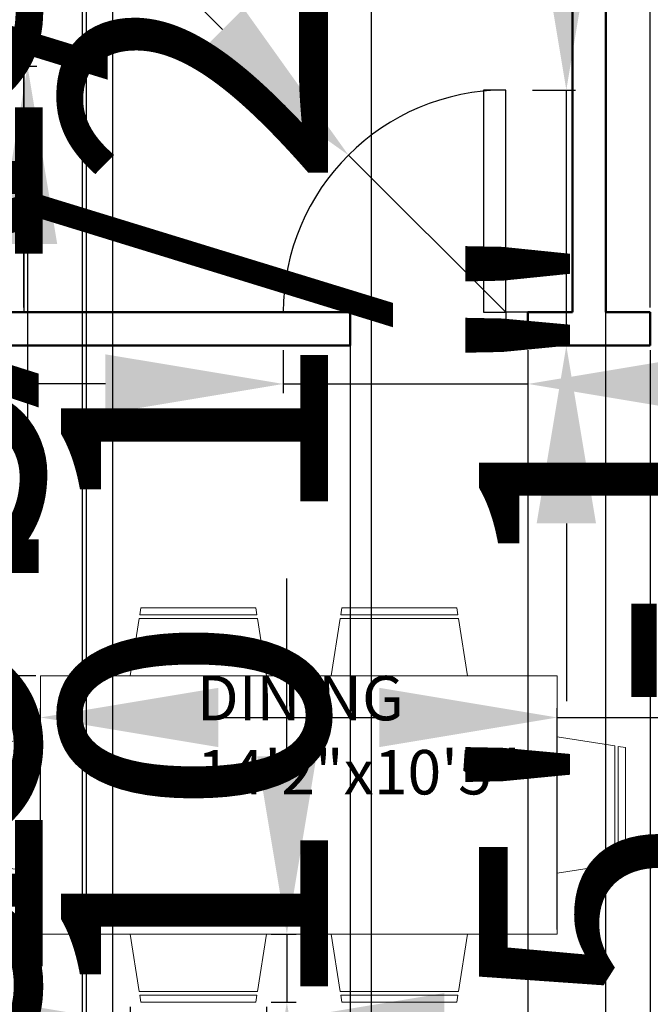
# Model space of a CAD drawing. Units: inches. Extents: x 1102 to 2414, y 295 to 1561.
# Tile 6 of 11: x 1610 to 1695, y 894 to 1027. Entities that reach past the tile are written whole.
import ezdxf

# ---------------------------------------------------------------- set-up
doc = ezdxf.new("R2010")
doc.units = ezdxf.units.IN
for name, color, linetype, lineweight in [('A-ANNO-DIMS', 2, 'Continuous', 18), ('A-AREA-IDEN', 7, 'Continuous', 25), ('A-DOOR', 4, 'Continuous', 25), ('A-FLOR-CASE', 8, 'Continuous', 25), ('A-FURN', 8, 'Continuous', 18), ('A-WALL', 7, 'Continuous', 50)]:
    doc.layers.add(name, color=color, linetype=linetype, lineweight=lineweight)
doc.styles.get("Standard").update_dxf_attribs({"font": 'arial.ttf'})
doc.dimstyles.new('ISO-25', dxfattribs={"dimtxt": 36, "dimasz": 24, "dimexe": 1.25, "dimexo": 0.625, "dimtad": 1, "dimlunit": 4, "dimtxsty": 'Standard', "dimcen": 2.5, "dimadec": 0, "dimazin": 0, "dimtfac": 1, "dimtmove": 0, "dimatfit": 3, "dimfxl": 1, "dimarcsym": 0})

# ---------------------------------------------------------------- blocks, each defined once
blk = doc.blocks.new('roomdoor')
for points in [[(1837.54, 1413.02), (1840.54, 1413.02), (1840.54, 1443.02), (1837.54, 1443.02)], [(1840.54, 1408.52), (1843.54, 1408.52), (1843.54, 1413.02), (1840.54, 1413.02)]]:
    blk.add_lwpolyline(points, close=True)
blk.add_arc((1840.54, 1413.02), 30, 90, 180)
blk = doc.blocks.new('CHAIR-DINING')
for p, q in [((1.44, 9.2), (1.29, 8.23)), ((17.08, 8.23), (1.29, 8.23)), ((1.44, 9.2), (16.93, 9.2)), ((17.08, 8.23), (16.93, 9.2)), ((1.21, 7.75), (0, 0)), ((1.21, 7.75), (17.16, 7.75)), ((18.37, 0), (17.16, 7.75))]:
    blk.add_line(p, q)
blk = doc.blocks.new('*D17')
at = {"layer": 'A-ANNO-DIMS', "color": 0, "lineweight": -2, "transparency": 16777216}
for p, q in [((1624.9, 893.98), (1624.9, 890.6)), ((1643.27, 893.98), (1643.27, 890.6)), ((1600.9, 891.85), (1102.3, 891.8)), ((1643.27, 891.85), (1624.9, 891.85)), ((1667.27, 891.85), (1691.27, 891.85))]:
    blk.add_line(p, q, dxfattribs=at)
at = {"layer": 'A-ANNO-DIMS', "color": 0, "transparency": 16777216}
for points in [[(1600.9, 895.85), (1600.9, 887.85), (1624.9, 891.85)], [(1667.27, 895.85), (1667.27, 887.85), (1643.27, 891.85)]]:
    blk.add_solid(points, dxfattribs=at)
at = {"layer": 'Defpoints', "color": 0, "transparency": 16777216}
for p in [(1624.9, 894.6), (1643.27, 894.6), (1624.9, 891.85)]:
    blk.add_point(p, dxfattribs=at)
at = {"layer": 'A-ANNO-DIMS', "color": 0, "transparency": 16777216, "insert": (1339.6, 911.06), "char_height": 36, "attachment_point": 5, "rotation": 0.0057}
blk.add_mtext('CHAIR 1\'-6 1/2" TYP.', dxfattribs=at)
blk = doc.blocks.new('*D18')
at = {"layer": 'A-ANNO-DIMS', "color": 0, "lineweight": -2, "transparency": 16777216}
for p, q in [((1646.02, 927.81), (1646.02, 951.81)), ((1643.89, 903.81), (1647.27, 903.81)), ((1646.02, 903.81), (1646.02, 894.61)), ((1643.89, 894.6), (1647.27, 894.61)), ((1646.03, 870.61), (1646.05, 625.92))]:
    blk.add_line(p, q, dxfattribs=at)
at = {"layer": 'A-ANNO-DIMS', "color": 0, "transparency": 16777216}
for points in [[(1650.02, 927.81), (1642.02, 927.81), (1646.02, 903.81)], [(1650.03, 870.61), (1642.03, 870.6), (1646.02, 894.61)]]:
    blk.add_solid(points, dxfattribs=at)
at = {"layer": 'Defpoints', "color": 0, "transparency": 16777216}
for p in [(1643.27, 903.81), (1643.27, 894.6), (1646.02, 894.61)]:
    blk.add_point(p, dxfattribs=at)
at = {"layer": 'A-ANNO-DIMS', "color": 0, "transparency": 16777216, "insert": (1665.05, 736.26), "char_height": 36, "attachment_point": 5, "rotation": 270.0057}
blk.add_mtext('0\'-9" TYP.', dxfattribs=at)
blk = doc.blocks.new('*D24')
at = {"layer": 'A-ANNO-DIMS', "color": 0, "lineweight": -2, "transparency": 16777216}
for p, q in [((1725.17, 1080.27), (1712.37, 1080.27)), ((1713.62, 1056.27), (1713.62, 1043.39)), ((1725.17, 1019.39), (1712.37, 1019.39)), ((1713.62, 1019.39), (1713.62, 898.44))]:
    blk.add_line(p, q, dxfattribs=at)
at = {"layer": 'A-ANNO-DIMS', "color": 0, "transparency": 16777216}
for points in [[(1709.62, 1056.27), (1717.62, 1056.27), (1713.62, 1080.27)], [(1709.62, 1043.39), (1717.62, 1043.39), (1713.62, 1019.39)]]:
    blk.add_solid(points, dxfattribs=at)
at = {"layer": 'Defpoints', "color": 0, "transparency": 16777216}
for p in [(1725.8, 1080.27), (1713.62, 1019.39), (1725.8, 1019.39)]:
    blk.add_point(p, dxfattribs=at)
at = {"layer": 'A-ANNO-DIMS', "color": 0, "transparency": 16777216, "insert": (1694.62, 946.91), "char_height": 36, "attachment_point": 5, "rotation": 90}
blk.add_mtext('5\'-1"', dxfattribs=at)
blk = doc.blocks.new('*D27')
at = {"layer": 'A-ANNO-DIMS', "color": 0, "lineweight": -2, "transparency": 16777216}
for p, q in [((1683.72, 1041.76), (1683.72, 1561.36)), ((1679.17, 1017.76), (1684.97, 1017.76)), ((1683.72, 983.26), (1683.72, 1017.76)), ((1679.17, 983.26), (1684.97, 983.26)), ((1683.72, 959.26), (1683.72, 935.26))]:
    blk.add_line(p, q, dxfattribs=at)
at = {"layer": 'A-ANNO-DIMS', "color": 0, "transparency": 16777216}
for points in [[(1679.72, 1041.76), (1687.72, 1041.76), (1683.72, 1017.76)], [(1679.72, 959.26), (1687.72, 959.26), (1683.72, 983.26)]]:
    blk.add_solid(points, dxfattribs=at)
at = {"layer": 'Defpoints', "color": 0, "transparency": 16777216}
for p in [(1678.54, 1017.76), (1683.72, 1017.76), (1678.54, 983.26)]:
    blk.add_point(p, dxfattribs=at)
at = {"layer": 'A-ANNO-DIMS', "color": 0, "transparency": 16777216, "insert": (1664.47, 1313.56), "char_height": 36, "attachment_point": 5, "rotation": 90}
blk.add_mtext('DOOR 2\'-10 1/2" TYP.', dxfattribs=at)
blk = doc.blocks.new('*D28')
at = {"layer": 'A-ANNO-DIMS', "color": 0, "lineweight": -2, "transparency": 16777216}
for p, q in [((1645.54, 982.63), (1645.54, 976.83)), ((1678.54, 982.63), (1678.54, 976.83)), ((1621.54, 978.08), (1597.54, 978.08)), ((1645.54, 978.08), (1678.54, 978.08)), ((1702.54, 978.08), (1947.85, 978.08))]:
    blk.add_line(p, q, dxfattribs=at)
at = {"layer": 'A-ANNO-DIMS', "color": 0, "transparency": 16777216}
for points in [[(1621.54, 982.08), (1621.54, 974.08), (1645.54, 978.08)], [(1702.54, 982.08), (1702.54, 974.08), (1678.54, 978.08)]]:
    blk.add_solid(points, dxfattribs=at)
at = {"layer": 'Defpoints', "color": 0, "transparency": 16777216}
for p in [(1645.54, 983.26), (1678.54, 983.26), (1678.54, 978.08)]:
    blk.add_point(p, dxfattribs=at)
at = {"layer": 'A-ANNO-DIMS', "color": 0, "transparency": 16777216, "insert": (1837.19, 997.09), "char_height": 36, "attachment_point": 5}
blk.add_mtext('2\'-9" TYP.', dxfattribs=at)
blk = doc.blocks.new('*D29')
at = {"layer": 'A-ANNO-DIMS', "color": 0, "lineweight": -2, "transparency": 16777216}
for p, q in [((1806.82, 1011.76), (1806.82, 1035.76)), ((1803.17, 987.76), (1808.07, 987.76)), ((1806.82, 987.76), (1806.82, 959.26)), ((1803.17, 959.26), (1808.07, 959.26)), ((1806.82, 935.26), (1806.82, 295.33))]:
    blk.add_line(p, q, dxfattribs=at)
at = {"layer": 'A-ANNO-DIMS', "color": 0, "transparency": 16777216}
for points in [[(1802.82, 1011.76), (1810.82, 1011.76), (1806.82, 987.76)], [(1802.82, 935.26), (1810.82, 935.26), (1806.82, 959.26)]]:
    blk.add_solid(points, dxfattribs=at)
at = {"layer": 'Defpoints', "color": 0, "transparency": 16777216}
for p in [(1802.54, 987.76), (1802.54, 959.26), (1806.82, 959.26)]:
    blk.add_point(p, dxfattribs=at)
at = {"layer": 'A-ANNO-DIMS', "color": 0, "transparency": 16777216, "insert": (1787.57, 603.3), "char_height": 36, "attachment_point": 5, "rotation": 90}
blk.add_mtext('BATH DOOR 2\'-4 1/2" TYP.', dxfattribs=at)
blk = doc.blocks.new('*D31')
at = {"layer": 'A-ANNO-DIMS', "color": 0, "lineweight": -2, "transparency": 16777216}
for p, q in [((1629.86, 764.63), (1629.86, 760.41)), ((1653.86, 764.63), (1653.86, 760.41)), ((1605.86, 761.66), (1581.86, 761.66)), ((1629.86, 761.66), (1653.86, 761.66)), ((1677.86, 761.66), (2225.36, 761.66))]:
    blk.add_line(p, q, dxfattribs=at)
at = {"layer": 'A-ANNO-DIMS', "color": 0, "transparency": 16777216}
for points in [[(1605.86, 765.66), (1605.86, 757.66), (1629.86, 761.66)], [(1677.86, 765.66), (1677.86, 757.66), (1653.86, 761.66)]]:
    blk.add_solid(points, dxfattribs=at)
at = {"layer": 'Defpoints', "color": 0, "transparency": 16777216}
for p in [(1629.86, 765.26), (1653.86, 765.26), (1653.86, 761.66)]:
    blk.add_point(p, dxfattribs=at)
at = {"layer": 'A-ANNO-DIMS', "color": 0, "transparency": 16777216, "insert": (1963.61, 780.91), "char_height": 36, "attachment_point": 5}
blk.add_mtext('DOOR LEAF 2\'-0" TYP.', dxfattribs=at)
blk = doc.blocks.new('*D32')
at = {"layer": 'A-ANNO-DIMS', "color": 0, "lineweight": -2, "transparency": 16777216}
for p, q in [((1657.46, 811.76), (1657.46, 1164.91)), ((1654.49, 787.76), (1658.71, 787.76)), ((1657.46, 765.26), (1657.46, 787.76)), ((1654.49, 765.26), (1658.71, 765.26)), ((1657.46, 741.26), (1657.46, 717.26))]:
    blk.add_line(p, q, dxfattribs=at)
at = {"layer": 'A-ANNO-DIMS', "color": 0, "transparency": 16777216}
for points in [[(1653.46, 811.76), (1661.46, 811.76), (1657.46, 787.76)], [(1653.46, 741.26), (1661.46, 741.26), (1657.46, 765.26)]]:
    blk.add_solid(points, dxfattribs=at)
at = {"layer": 'Defpoints', "color": 0, "transparency": 16777216}
for p in [(1653.86, 787.76), (1657.46, 787.76), (1653.86, 765.26)]:
    blk.add_point(p, dxfattribs=at)
at = {"layer": 'A-ANNO-DIMS', "color": 0, "transparency": 16777216, "insert": (1638.22, 1000.34), "char_height": 36, "attachment_point": 5, "rotation": 90}
blk.add_mtext('1\'-10 1/2" TYP.', dxfattribs=at)
blk = doc.blocks.new('*D35')
at = {"layer": 'A-ANNO-DIMS', "color": 0, "lineweight": -2, "transparency": 16777216}
for p, q in [((1611.04, 1074.99), (1611.04, 1327.12)), ((1607.17, 1050.99), (1612.29, 1050.99)), ((1611.04, 1020.99), (1611.04, 1050.99)), ((1607.17, 1020.99), (1612.29, 1020.99)), ((1611.04, 996.99), (1611.04, 972.99))]:
    blk.add_line(p, q, dxfattribs=at)
at = {"layer": 'A-ANNO-DIMS', "color": 0, "transparency": 16777216}
for points in [[(1607.04, 1074.99), (1615.04, 1074.99), (1611.04, 1050.99)], [(1607.04, 996.99), (1615.04, 996.99), (1611.04, 1020.99)]]:
    blk.add_solid(points, dxfattribs=at)
at = {"layer": 'Defpoints', "color": 0, "transparency": 16777216}
for p in [(1606.54, 1050.99), (1611.04, 1050.99), (1606.54, 1020.99)]:
    blk.add_point(p, dxfattribs=at)
at = {"layer": 'A-ANNO-DIMS', "color": 0, "transparency": 16777216, "insert": (1591.81, 1213.06), "char_height": 36, "attachment_point": 5, "rotation": 90}
blk.add_mtext('SINK 2\'-6"', dxfattribs=at)
blk = doc.blocks.new('*D37')
at = {"layer": 'A-ANNO-DIMS', "color": 0, "lineweight": -2, "transparency": 16777216}
for p, q in [((1618.46, 855.15), (1618.46, 1126.82)), ((1612.94, 831.15), (1619.71, 831.15)), ((1618.46, 790.23), (1618.46, 831.15)), ((1612.94, 790.23), (1619.71, 790.23)), ((1618.46, 766.23), (1618.46, 742.23))]:
    blk.add_line(p, q, dxfattribs=at)
at = {"layer": 'A-ANNO-DIMS', "color": 0, "transparency": 16777216}
for points in [[(1614.46, 855.15), (1622.46, 855.15), (1618.46, 831.15)], [(1614.46, 766.23), (1622.46, 766.23), (1618.46, 790.23)]]:
    blk.add_solid(points, dxfattribs=at)
at = {"layer": 'Defpoints', "color": 0, "transparency": 16777216}
for p in [(1612.32, 831.15), (1618.46, 831.15), (1612.32, 790.23)]:
    blk.add_point(p, dxfattribs=at)
at = {"layer": 'A-ANNO-DIMS', "color": 0, "transparency": 16777216, "insert": (1599.19, 1002.98), "char_height": 36, "attachment_point": 5, "rotation": 90}
blk.add_mtext('SOFA 3\'-5"', dxfattribs=at)
blk = doc.blocks.new('*D39')
at = {"layer": 'A-ANNO-DIMS', "color": 0, "lineweight": -2, "transparency": 16777216}
for p, q in [((1623.32, 855.67), (1623.32, 860.64)), ((1652.27, 855.67), (1652.27, 860.64)), ((1599.32, 859.39), (1575.32, 859.39)), ((1623.32, 859.39), (1652.27, 859.39)), ((1676.27, 859.39), (2075.12, 859.39))]:
    blk.add_line(p, q, dxfattribs=at)
at = {"layer": 'A-ANNO-DIMS', "color": 0, "transparency": 16777216}
for points in [[(1599.32, 863.39), (1599.32, 855.39), (1623.32, 859.39)], [(1676.27, 863.39), (1676.27, 855.39), (1652.27, 859.39)]]:
    blk.add_solid(points, dxfattribs=at)
at = {"layer": 'Defpoints', "color": 0, "transparency": 16777216}
for p in [(1652.27, 859.39), (1623.32, 855.05), (1652.27, 855.05)]:
    blk.add_point(p, dxfattribs=at)
at = {"layer": 'A-ANNO-DIMS', "color": 0, "transparency": 16777216, "insert": (1887.69, 878.64), "char_height": 36, "attachment_point": 5}
blk.add_mtext('LOVESEAT 2\'-5"', dxfattribs=at)
blk = doc.blocks.new('*D40')
at = {"layer": 'A-ANNO-DIMS', "color": 0, "lineweight": -2, "transparency": 16777216}
for p, q in [((1618.98, 879.05), (1618.98, 1080.49)), ((1622.7, 855.05), (1617.73, 855.05)), ((1618.98, 837.36), (1618.98, 855.05)), ((1622.7, 837.36), (1617.73, 837.36)), ((1618.98, 813.36), (1618.98, 789.36))]:
    blk.add_line(p, q, dxfattribs=at)
at = {"layer": 'A-ANNO-DIMS', "color": 0, "transparency": 16777216}
for points in [[(1614.98, 879.05), (1622.98, 879.05), (1618.98, 855.05)], [(1614.98, 813.36), (1622.98, 813.36), (1618.98, 837.36)]]:
    blk.add_solid(points, dxfattribs=at)
at = {"layer": 'Defpoints', "color": 0, "transparency": 16777216}
for p in [(1618.98, 855.05), (1623.32, 855.05), (1623.32, 837.36)]:
    blk.add_point(p, dxfattribs=at)
at = {"layer": 'A-ANNO-DIMS', "color": 0, "transparency": 16777216, "insert": (1599.74, 991.77), "char_height": 36, "attachment_point": 5, "rotation": 90}
blk.add_mtext('1\'-5 1/2"', dxfattribs=at)
blk = doc.blocks.new('*D45')
at = {"layer": 'A-ANNO-DIMS', "color": 0, "lineweight": -2, "transparency": 16777216}
for p, q in [((1736.54, 770.38), (1736.54, 1147.26)), ((1754.54, 770.38), (1754.54, 1147.26)), ((1712.54, 1146.01), (1688.54, 1146.01)), ((1736.54, 1146.01), (1754.54, 1146.01)), ((1778.54, 1146.01), (1896.1, 1146.01))]:
    blk.add_line(p, q, dxfattribs=at)
at = {"layer": 'A-ANNO-DIMS', "color": 0, "transparency": 16777216}
for points in [[(1712.54, 1150.01), (1712.54, 1142.01), (1736.54, 1146.01)], [(1778.54, 1150.01), (1778.54, 1142.01), (1754.54, 1146.01)]]:
    blk.add_solid(points, dxfattribs=at)
at = {"layer": 'Defpoints', "color": 0, "transparency": 16777216}
for p in [(1754.54, 1146.01), (1736.54, 769.76), (1754.54, 769.76)]:
    blk.add_point(p, dxfattribs=at)
at = {"layer": 'A-ANNO-DIMS', "color": 0, "transparency": 16777216, "insert": (1849.32, 1165.02), "char_height": 36, "attachment_point": 5}
blk.add_mtext('1\'-6"', dxfattribs=at)
blk = doc.blocks.new('*D48')
at = {"layer": 'A-ANNO-DIMS', "color": 0, "lineweight": -2, "transparency": 16777216}
for p, q in [((1689.04, 854.38), (1689.04, 1147.26)), ((1732.04, 858.88), (1732.04, 1147.26)), ((1665.04, 1146.01), (1641.04, 1146.01)), ((1689.04, 1146.01), (1732.04, 1146.01)), ((1756.04, 1146.01), (1876.97, 1146.01))]:
    blk.add_line(p, q, dxfattribs=at)
at = {"layer": 'A-ANNO-DIMS', "color": 0, "transparency": 16777216}
for points in [[(1665.04, 1150.01), (1665.04, 1142.01), (1689.04, 1146.01)], [(1756.04, 1150.01), (1756.04, 1142.01), (1732.04, 1146.01)]]:
    blk.add_solid(points, dxfattribs=at)
at = {"layer": 'Defpoints', "color": 0, "transparency": 16777216}
for p in [(1732.04, 1146.01), (1732.04, 858.26), (1689.04, 853.76)]:
    blk.add_point(p, dxfattribs=at)
at = {"layer": 'A-ANNO-DIMS', "color": 0, "transparency": 16777216, "insert": (1828.51, 1165.03), "char_height": 36, "attachment_point": 5}
blk.add_mtext('3\'-7"', dxfattribs=at)
blk = doc.blocks.new('*D50')
at = {"layer": 'A-ANNO-DIMS', "color": 0, "lineweight": -2, "transparency": 16777216}
for p, q in [((1586.54, 987.13), (1586.54, 606.26)), ((1654.54, 987.13), (1654.54, 606.26)), ((1610.54, 607.51), (1630.54, 607.51)), ((1654.54, 607.51), (1775.49, 607.51))]:
    blk.add_line(p, q, dxfattribs=at)
at = {"layer": 'A-ANNO-DIMS', "color": 0, "transparency": 16777216}
for points in [[(1610.54, 611.51), (1610.54, 603.51), (1586.54, 607.51)], [(1630.54, 611.51), (1630.54, 603.51), (1654.54, 607.51)]]:
    blk.add_solid(points, dxfattribs=at)
at = {"layer": 'Defpoints', "color": 0, "transparency": 16777216}
for p in [(1586.54, 987.76), (1654.54, 987.76), (1654.54, 607.51)]:
    blk.add_point(p, dxfattribs=at)
at = {"layer": 'A-ANNO-DIMS', "color": 0, "transparency": 16777216, "insert": (1727.02, 626.52), "char_height": 36, "attachment_point": 5}
blk.add_mtext('5\'-8"', dxfattribs=at)
blk = doc.blocks.new('*D51')
at = {"layer": 'A-ANNO-DIMS', "color": 0, "lineweight": -2, "transparency": 16777216}
for p, q in [((1689.04, 988.38), (1689.04, 1147.26)), ((1695.04, 988.38), (1695.04, 1147.26)), ((1665.04, 1146.01), (1641.04, 1146.01)), ((1689.04, 1146.01), (1695.04, 1146.01)), ((1719.04, 1146.01), (1839.99, 1146.01))]:
    blk.add_line(p, q, dxfattribs=at)
at = {"layer": 'A-ANNO-DIMS', "color": 0, "transparency": 16777216}
for points in [[(1665.04, 1150.01), (1665.04, 1142.01), (1689.04, 1146.01)], [(1719.04, 1150.01), (1719.04, 1142.01), (1695.04, 1146.01)]]:
    blk.add_solid(points, dxfattribs=at)
at = {"layer": 'Defpoints', "color": 0, "transparency": 16777216}
for p in [(1695.04, 1146.01), (1689.04, 987.76), (1695.04, 987.76)]:
    blk.add_point(p, dxfattribs=at)
at = {"layer": 'A-ANNO-DIMS', "color": 0, "transparency": 16777216, "insert": (1791.52, 1165.02), "char_height": 36, "attachment_point": 5}
blk.add_mtext('0\'-6"', dxfattribs=at)
blk = doc.blocks.new('*D53')
at = {"layer": 'A-ANNO-DIMS', "color": 0, "lineweight": -2, "transparency": 16777216}
for p, q in [((1586.54, 988.38), (1586.54, 1147.26)), ((1610.54, 988.38), (1610.54, 1147.26)), ((1562.54, 1146.01), (1538.54, 1146.01)), ((1586.54, 1146.01), (1610.54, 1146.01)), ((1634.54, 1146.01), (1756.11, 1146.01))]:
    blk.add_line(p, q, dxfattribs=at)
at = {"layer": 'A-ANNO-DIMS', "color": 0, "transparency": 16777216}
for points in [[(1562.54, 1150.01), (1562.54, 1142.01), (1586.54, 1146.01)], [(1634.54, 1150.01), (1634.54, 1142.01), (1610.54, 1146.01)]]:
    blk.add_solid(points, dxfattribs=at)
at = {"layer": 'Defpoints', "color": 0, "transparency": 16777216}
for p in [(1610.54, 1146.01), (1586.54, 987.76), (1610.54, 987.76)]:
    blk.add_point(p, dxfattribs=at)
at = {"layer": 'A-ANNO-DIMS', "color": 0, "transparency": 16777216, "insert": (1707.32, 1165.02), "char_height": 36, "attachment_point": 5}
blk.add_mtext('2\'-0"', dxfattribs=at)
blk = doc.blocks.new('*D55')
at = {"layer": 'A-ANNO-DIMS', "color": 0, "lineweight": -2, "transparency": 16777216}
for p, q in [((1586.54, 722.38), (1586.54, 1147.26)), ((1622.54, 722.38), (1622.54, 1147.26)), ((1562.54, 1146.01), (1538.54, 1146.01)), ((1586.54, 1146.01), (1622.54, 1146.01)), ((1646.54, 1146.01), (1767.47, 1146.01))]:
    blk.add_line(p, q, dxfattribs=at)
at = {"layer": 'A-ANNO-DIMS', "color": 0, "transparency": 16777216}
for points in [[(1562.54, 1150.01), (1562.54, 1142.01), (1586.54, 1146.01)], [(1646.54, 1150.01), (1646.54, 1142.01), (1622.54, 1146.01)]]:
    blk.add_solid(points, dxfattribs=at)
at = {"layer": 'Defpoints', "color": 0, "transparency": 16777216}
for p in [(1622.54, 1146.01), (1586.54, 721.76), (1622.54, 721.76)]:
    blk.add_point(p, dxfattribs=at)
at = {"layer": 'A-ANNO-DIMS', "color": 0, "transparency": 16777216, "insert": (1719.01, 1165.03), "char_height": 36, "attachment_point": 5}
blk.add_mtext('3\'-0"', dxfattribs=at)
blk = doc.blocks.new('*D58')
at = {"layer": 'A-ANNO-DIMS', "color": 0, "lineweight": -2, "transparency": 16777216}
for p, q in [((1612.78, 904.43), (1612.78, 934.3)), ((1682.5, 904.43), (1682.5, 934.3)), ((1636.78, 933.05), (1658.5, 933.05)), ((1682.5, 933.05), (1887.33, 933.05))]:
    blk.add_line(p, q, dxfattribs=at)
at = {"layer": 'A-ANNO-DIMS', "color": 0, "transparency": 16777216}
for points in [[(1636.78, 937.05), (1636.78, 929.05), (1612.78, 933.05)], [(1658.5, 937.05), (1658.5, 929.05), (1682.5, 933.05)]]:
    blk.add_solid(points, dxfattribs=at)
at = {"layer": 'Defpoints', "color": 0, "transparency": 16777216}
for p in [(1682.5, 933.05), (1612.78, 903.8), (1682.5, 903.8)]:
    blk.add_point(p, dxfattribs=at)
at = {"layer": 'A-ANNO-DIMS', "color": 0, "transparency": 16777216, "insert": (1796.92, 952.29), "char_height": 36, "attachment_point": 5}
blk.add_mtext('5\'-9 1/2"', dxfattribs=at)
blk = doc.blocks.new('*D59')
at = {"layer": 'A-ANNO-DIMS', "color": 0, "lineweight": -2, "transparency": 16777216}
for p, q in [((1548.29, 962.66), (1548.29, 1112.19)), ((1612.15, 938.66), (1547.04, 938.66)), ((1548.29, 903.8), (1548.29, 938.66)), ((1612.15, 903.8), (1547.04, 903.8)), ((1548.29, 879.8), (1548.29, 855.8))]:
    blk.add_line(p, q, dxfattribs=at)
at = {"layer": 'A-ANNO-DIMS', "color": 0, "transparency": 16777216}
for points in [[(1544.29, 962.66), (1552.29, 962.66), (1548.29, 938.66)], [(1544.29, 879.8), (1552.29, 879.8), (1548.29, 903.8)]]:
    blk.add_solid(points, dxfattribs=at)
at = {"layer": 'Defpoints', "color": 0, "transparency": 16777216}
for p in [(1548.29, 938.66), (1612.78, 938.66), (1612.78, 903.8)]:
    blk.add_point(p, dxfattribs=at)
at = {"layer": 'A-ANNO-DIMS', "color": 0, "transparency": 16777216, "insert": (1529.6, 1049.43), "char_height": 36, "attachment_point": 5, "rotation": 90}
blk.add_mtext('2\'-11"', dxfattribs=at)
blk = doc.blocks.new('*D63')
at = {"layer": 'A-ANNO-DIMS', "color": 0, "lineweight": -2, "transparency": 16777216}
for p, q in [((1654.54, 982.63), (1654.54, 606.26)), ((1678.54, 982.63), (1678.54, 606.26)), ((1630.54, 607.51), (1606.54, 607.51)), ((1654.54, 607.51), (1678.54, 607.51)), ((1702.54, 607.51), (1824.11, 607.51))]:
    blk.add_line(p, q, dxfattribs=at)
at = {"layer": 'A-ANNO-DIMS', "color": 0, "transparency": 16777216}
for points in [[(1630.54, 611.51), (1630.54, 603.51), (1654.54, 607.51)], [(1702.54, 611.51), (1702.54, 603.51), (1678.54, 607.51)]]:
    blk.add_solid(points, dxfattribs=at)
at = {"layer": 'Defpoints', "color": 0, "transparency": 16777216}
for p in [(1654.54, 983.26), (1678.54, 983.26), (1678.54, 607.51)]:
    blk.add_point(p, dxfattribs=at)
at = {"layer": 'A-ANNO-DIMS', "color": 0, "transparency": 16777216, "insert": (1775.32, 626.52), "char_height": 36, "attachment_point": 5}
blk.add_mtext('2\'-0"', dxfattribs=at)
blk = doc.blocks.new('*D64')
at = {"layer": 'A-ANNO-DIMS', "color": 0, "lineweight": -2, "transparency": 16777216}
for p, q in [((1695.04, 982.63), (1695.04, 606.26)), ((1719.04, 982.63), (1719.04, 606.26)), ((1671.04, 607.51), (1647.04, 607.51)), ((1695.04, 607.51), (1719.04, 607.51)), ((1743.04, 607.51), (1864.61, 607.51))]:
    blk.add_line(p, q, dxfattribs=at)
at = {"layer": 'A-ANNO-DIMS', "color": 0, "transparency": 16777216}
for points in [[(1671.04, 611.51), (1671.04, 603.51), (1695.04, 607.51)], [(1743.04, 611.51), (1743.04, 603.51), (1719.04, 607.51)]]:
    blk.add_solid(points, dxfattribs=at)
at = {"layer": 'Defpoints', "color": 0, "transparency": 16777216}
for p in [(1695.04, 983.26), (1719.04, 983.26), (1719.04, 607.51)]:
    blk.add_point(p, dxfattribs=at)
at = {"layer": 'A-ANNO-DIMS', "color": 0, "transparency": 16777216, "insert": (1815.82, 626.52), "char_height": 36, "attachment_point": 5}
blk.add_mtext('2\'-0"', dxfattribs=at)
blk = doc.blocks.new('*D65')
at = {"layer": 'A-ANNO-DIMS', "color": 0, "lineweight": -2, "transparency": 16777216}
for p, q in [((1697.64, 770.38), (1697.64, 1147.26)), ((1725.04, 770.38), (1725.04, 1147.26)), ((1673.64, 1146.01), (1649.64, 1146.01)), ((1697.64, 1146.01), (1725.04, 1146.01)), ((1749.04, 1146.01), (1954.49, 1146.01))]:
    blk.add_line(p, q, dxfattribs=at)
at = {"layer": 'A-ANNO-DIMS', "color": 0, "transparency": 16777216}
for points in [[(1673.64, 1150.01), (1673.64, 1142.01), (1697.64, 1146.01)], [(1749.04, 1150.01), (1749.04, 1142.01), (1725.04, 1146.01)]]:
    blk.add_solid(points, dxfattribs=at)
at = {"layer": 'Defpoints', "color": 0, "transparency": 16777216}
for p in [(1725.04, 1146.01), (1697.64, 769.76), (1725.04, 769.76)]:
    blk.add_point(p, dxfattribs=at)
at = {"layer": 'A-ANNO-DIMS', "color": 0, "transparency": 16777216, "insert": (1863.77, 1165.26), "char_height": 36, "attachment_point": 5}
blk.add_mtext('2\'-3 1/2"', dxfattribs=at)
blk = doc.blocks.new('*D68')
at = {"layer": 'A-ANNO-DIMS', "color": 0, "lineweight": -2, "transparency": 16777216}
for p, q in [((1527.48, 1135.83), (1637.36, 1025.94)), ((1675.54, 987.76), (1654.33, 1008.97))]:
    blk.add_line(p, q, dxfattribs=at)
at = {"layer": 'A-ANNO-DIMS', "color": 0, "transparency": 16777216}
blk.add_solid([(1640.19, 1028.77), (1634.53, 1023.12), (1654.33, 1008.97)], dxfattribs=at)
at = {"layer": 'Defpoints', "color": 0, "transparency": 16777216}
for p in [(1654.33, 1008.97), (1675.54, 987.76)]:
    blk.add_point(p, dxfattribs=at)
at = {"layer": 'A-ANNO-DIMS', "color": 0, "transparency": 16777216, "insert": (1587.37, 1102.81), "char_height": 36, "attachment_point": 5, "rotation": 314.9996}
blk.add_mtext('R2\'-6"', dxfattribs=at)
blk = doc.blocks.new('*D69')
at = {"layer": 'A-ANNO-DIMS', "color": 0, "lineweight": -2, "transparency": 16777216}
for p, q in [((1775.45, 909.34), (1665.56, 799.46)), ((1635.86, 769.76), (1648.59, 782.49))]:
    blk.add_line(p, q, dxfattribs=at)
at = {"layer": 'A-ANNO-DIMS', "color": 0, "transparency": 16777216}
blk.add_solid([(1662.73, 802.29), (1668.39, 796.63), (1648.59, 782.49)], dxfattribs=at)
at = {"layer": 'Defpoints', "color": 0, "transparency": 16777216}
for p in [(1648.59, 782.49), (1635.86, 769.76)]:
    blk.add_point(p, dxfattribs=at)
at = {"layer": 'A-ANNO-DIMS', "color": 0, "transparency": 16777216, "insert": (1715.55, 876.32), "char_height": 36, "attachment_point": 5, "rotation": 45}
blk.add_mtext('R1\'-6"', dxfattribs=at)

msp = doc.modelspace()

# ---------------------------------------------------------------- linework, layer by layer
at = {"layer": 'A-FLOR-CASE'}
msp.add_line((1610.544, 1079.395), (1610.544, 987.76), dxfattribs=at)
at = {"layer": 'A-FURN'}
for p, q in [((1682.499, 938.663), (1612.778, 938.663)), ((1612.778, 938.663), (1612.778, 903.803)), ((1682.499, 903.803), (1682.499, 938.663)), ((1612.778, 903.803), (1682.499, 903.803))]:
    msp.add_line(p, q, dxfattribs=at)
at = {"layer": 'A-WALL'}
for p, q in [((1684.544, 1107.76), (1684.544, 987.76)), ((1689.044, 1107.76), (1689.044, 987.76)), ((1654.544, 987.76), (1586.544, 987.76)), ((1654.544, 987.76), (1654.544, 983.26)), ((1684.544, 987.76), (1678.544, 987.76)), ((1684.544, 987.76), (1678.544, 987.76)), ((1678.544, 987.76), (1678.544, 983.26)), ((1689.044, 987.76), (1695.044, 987.76)), ((1695.044, 987.76), (1689.044, 987.76)), ((1695.044, 987.76), (1695.044, 983.26)), ((1654.544, 983.26), (1586.544, 983.26)), ((1689.044, 983.26), (1678.544, 983.26)), ((1695.044, 983.26), (1689.044, 983.26))]:
    msp.add_line(p, q, dxfattribs=at)

# ---------------------------------------------------------------- block references
at = {"layer": 'A-DOOR'}
msp.add_blockref('roomdoor', (-165, -425.258), dxfattribs=at)
at = {"layer": 'A-FURN'}
for p in [(1624.897, 938.661), (1652.011, 938.661)]:
    msp.add_blockref('CHAIR-DINING', p, dxfattribs=at)
for p, rotation in [((1612.782, 912.048), 90.00584970642711), ((1682.497, 930.418), 269.9999986166272), ((1643.268, 903.806), 180.0056718243519), ((1670.381, 903.806), 180.0056718243519)]:
    msp.add_blockref('CHAIR-DINING', p, dxfattribs=dict(at, rotation=rotation))

# ---------------------------------------------------------------- texts
at = {"layer": 'A-AREA-IDEN', "insert": (1633.895, 938.663), "char_height": 6, "attachment_point": 1}
msp.add_mtext_dynamic_manual_height_columns('DINING\\P14\'2"x10\'5"', width=50.64919, gutter_width=12.5, heights=[0], dxfattribs=at)

# ---------------------------------------------------------------- dimensions: what is measured, and where the dimension line sits
at = {"layer": 'A-ANNO-DIMS'}
for base, p1, p2, angle, text, picture, middle in [((1683.719, 1017.76), (1678.544, 983.26), (1678.544, 1017.76), 90, 'DOOR <> TYP.', '*D27', (1664.468, 1313.559)), ((1611.044, 1050.991), (1606.544, 1020.991), (1606.544, 1050.991), 90, 'SINK <>', '*D35', (1591.805, 1213.055)), ((1657.464, 787.76), (1653.864, 765.26), (1653.864, 787.76), 90, '<> TYP.', '*D32', (1638.225, 1000.337)), ((1618.456, 831.145), (1612.319, 790.233), (1612.319, 831.145), 90, 'SOFA <>', '*D37', (1599.192, 1002.983)), ((1806.819, 959.26), (1802.544, 987.76), (1802.544, 959.26), 270, 'BATH DOOR <> TYP.', '*D29', (1787.568, 603.296)), ((1624.9, 891.848), (1643.269, 894.605), (1624.9, 894.603), 180.00567, 'CHAIR <> TYP.', '*D17', (1339.596, 911.058)), ((1646.024, 894.605), (1643.268, 903.806), (1643.269, 894.605), 270.00567, '<> TYP.', '*D18', (1665.045, 736.263))]:
    dim = msp.add_linear_dim(base=base, p1=p1, p2=p2, angle=angle, text=text, dimstyle='ISO-25', override={"dimdec": 1, "dimlfac": 1, "dimrnd": 0, "dimzin": 1, "dimdsep": 46, "dimlunit": 4, "dimfrac": 2}, dxfattribs=at)
    dim.commit()
    dim.dimension.update_dxf_attribs({"geometry": picture, "text_midpoint": middle})
for base, p1, p2, picture, middle in [((1725.044, 1146.01), (1697.644, 769.76), (1725.044, 769.76), '*D65', (1863.767, 1165.261)), ((1622.544, 1146.01), (1586.544, 721.76), (1622.544, 721.76), '*D55', (1719.005, 1165.028)), ((1610.544, 1146.01), (1586.544, 987.76), (1610.544, 987.76), '*D53', (1707.325, 1165.015)), ((1732.044, 1146.01), (1689.044, 853.76), (1732.044, 858.26), '*D48', (1828.505, 1165.028)), ((1695.044, 1146.01), (1689.044, 987.76), (1695.044, 987.76), '*D51', (1791.518, 1165.015)), ((1754.544, 1146.01), (1736.544, 769.76), (1754.544, 769.76), '*D45', (1849.323, 1165.015)), ((1682.499, 933.053), (1612.778, 903.803), (1682.499, 903.803), '*D58', (1796.915, 952.292)), ((1654.544, 607.51), (1586.544, 987.76), (1654.544, 987.76), '*D50', (1727.018, 626.515)), ((1678.544, 607.51), (1654.544, 983.26), (1678.544, 983.26), '*D63', (1775.325, 626.515)), ((1719.044, 607.51), (1695.044, 983.26), (1719.044, 983.26), '*D64', (1815.825, 626.515))]:
    dim = msp.add_linear_dim(base=base, p1=p1, p2=p2, dimstyle='ISO-25', override={"dimdec": 1, "dimlfac": 1, "dimrnd": 0, "dimzin": 1, "dimdsep": 46, "dimlunit": 4, "dimfrac": 2}, dxfattribs=at)
    dim.commit()
    dim.dimension.update_dxf_attribs({"geometry": picture, "text_midpoint": middle})
for center, mpoint, picture, middle in [((1675.544, 987.76), (1654.331, 1008.973), '*D68', (1587.373, 1102.811)), ((1635.864, 769.76), (1648.592, 782.488), '*D69', (1715.551, 876.325))]:
    dim = msp.add_radius_dim(center=center, mpoint=mpoint, dimstyle='ISO-25', override={"dimdec": 1, "dimlfac": 1, "dimrnd": 0, "dimzin": 1, "dimdsep": 46, "dimlunit": 4, "dimfrac": 2}, dxfattribs=at)
    dim.commit()
    dim.dimension.update_dxf_attribs({"geometry": picture, "text_midpoint": middle})
for base, p1, p2, angle, picture, middle in [((1548.294, 938.663), (1612.778, 903.803), (1612.778, 938.663), 90, '*D59', (1529.595, 1049.429)), ((1618.978, 855.046), (1623.32, 837.356), (1623.32, 855.046), 90, '*D40', (1599.739, 991.768)), ((1713.621, 1019.387), (1725.798, 1080.268), (1725.798, 1019.387), 270, '*D24', (1694.616, 946.913))]:
    dim = msp.add_linear_dim(base=base, p1=p1, p2=p2, angle=angle, dimstyle='ISO-25', override={"dimdec": 1, "dimlfac": 1, "dimrnd": 0, "dimzin": 1, "dimdsep": 46, "dimlunit": 4, "dimfrac": 2}, dxfattribs=at)
    dim.commit()
    dim.dimension.update_dxf_attribs({"geometry": picture, "text_midpoint": middle})
for base, p1, p2, text, picture, middle in [((1678.544, 978.085), (1645.544, 983.26), (1678.544, 983.26), '<> TYP.', '*D28', (1837.195, 997.09)), ((1652.268, 859.388), (1623.32, 855.046), (1652.268, 855.046), 'LOVESEAT <>', '*D39', (1887.695, 878.64)), ((1653.864, 761.66), (1629.864, 765.26), (1653.864, 765.26), 'DOOR LEAF <> TYP.', '*D31', (1963.611, 780.911))]:
    dim = msp.add_linear_dim(base=base, p1=p1, p2=p2, text=text, dimstyle='ISO-25', override={"dimdec": 1, "dimlfac": 1, "dimrnd": 0, "dimzin": 1, "dimdsep": 46, "dimlunit": 4, "dimfrac": 2}, dxfattribs=at)
    dim.commit()
    dim.dimension.update_dxf_attribs({"geometry": picture, "text_midpoint": middle})

doc.saveas('drawing.dxf')
